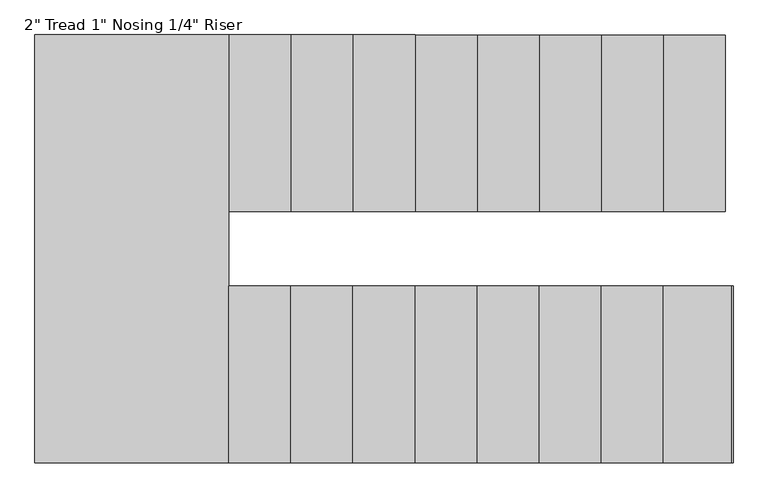
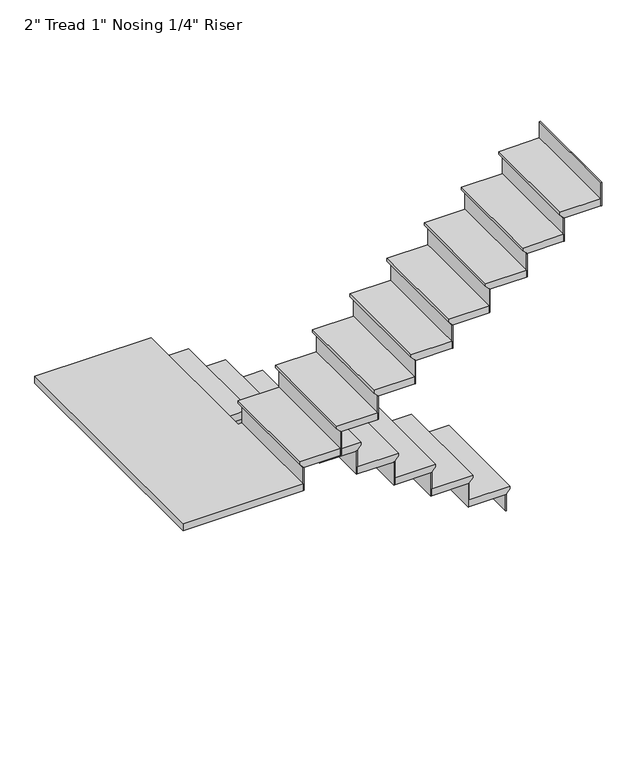
"""IFC4 building model written with IfcOpenShell, lengths in millimetres: stair flight geometry."""

from ifc_helpers import new_model, si_unit, origin, place, context, project, spatial, faceted_brep, source, transform, mapped, element, save


def stair_flight_94c6aef5(model_context):
    return source(origin(), model_context, "Body", "Brep", [
        faceted_brep([(-2118.1728655, 1192.5797121, 9292.8722222), (-2118.1728655, 1192.5797121, 9311.9222222), (-2118.1728655, 468.6797121, 9311.9222222), (-2118.1728655, 468.6797121, 9292.8722222), (-2143.5728655, 1192.5797121, 9267.4722222), (-2143.5728655, 468.6797121, 9267.4722222), (-2397.5728655, 1192.5797121, 9311.9222222), (-2397.5728655, 468.6797121, 9311.9222222), (-2143.5728655, 468.6797121, 9261.1222222), (-2397.5728655, 468.6797121, 9261.1222222), (-2397.5728655, 1192.5797121, 9261.1222222), (-2143.5728655, 1192.5797121, 9261.1222222)], [[[0, 1, 2, 3]], [[4, 0, 3, 5]], [[2, 1, 6, 7]], [[8, 9, 10, 11]], [[2, 7, 9, 8, 5, 3]], [[8, 11, 4, 5]], [[6, 1, 0, 4, 11, 10]], [[7, 6, 10, 9]]]),
        faceted_brep([(-2143.5728655, 1192.5797121, 9261.1222222), (-2143.5728655, 1192.5797121, 9144.0), (-2149.9228655, 1192.5797121, 9144.0), (-2149.9228655, 1192.5797121, 9261.1222222), (-2143.5728655, 468.6797121, 9261.1222222), (-2149.9228655, 468.6797121, 9261.1222222), (-2149.9228655, 468.6797121, 9144.0), (-2143.5728655, 468.6797121, 9144.0)], [[[0, 1, 2, 3]], [[4, 5, 6, 7]], [[1, 0, 4, 7]], [[2, 1, 7, 6]], [[3, 2, 6, 5]], [[0, 3, 5, 4]]]),
        faceted_brep([(-2397.5728655, 1192.5797121, 9429.0444444), (-2397.5728655, 1192.5797121, 9261.1222222), (-2403.9228655, 1192.5797121, 9261.1222222), (-2403.9228655, 1192.5797121, 9429.0444444), (-2397.5728655, 468.6797121, 9429.0444444), (-2403.9228655, 468.6797121, 9429.0444444), (-2403.9228655, 468.6797121, 9261.1222222), (-2397.5728655, 468.6797121, 9261.1222222)], [[[0, 1, 2, 3]], [[4, 5, 6, 7]], [[1, 0, 4, 7]], [[2, 1, 7, 6]], [[3, 2, 6, 5]], [[0, 3, 5, 4]]]),
        faceted_brep([(-2372.1728655, 468.6797121, 9479.8444444), (-2372.1728655, 1192.5797121, 9479.8444444), (-2651.5728655, 1192.5797121, 9479.8444444), (-2651.5728655, 468.6797121, 9479.8444444), (-2397.5728655, 468.6797121, 9429.0444444), (-2651.5728655, 468.6797121, 9429.0444444), (-2651.5728655, 1192.5797121, 9429.0444444), (-2397.5728655, 1192.5797121, 9429.0444444), (-2397.5728655, 468.6797121, 9435.3944444), (-2372.1728655, 468.6797121, 9460.7944444), (-2397.5728655, 1192.5797121, 9435.3944444), (-2372.1728655, 1192.5797121, 9460.7944444)], [[[0, 1, 2, 3]], [[4, 5, 6, 7]], [[0, 3, 5, 4, 8, 9]], [[4, 7, 10, 8]], [[2, 1, 11, 10, 7, 6]], [[3, 2, 6, 5]], [[11, 1, 0, 9]], [[10, 11, 9, 8]]]),
        faceted_brep([(-2651.5728655, 1192.5797121, 9596.9666667), (-2651.5728655, 1192.5797121, 9429.0444444), (-2657.9228655, 1192.5797121, 9429.0444444), (-2657.9228655, 1192.5797121, 9596.9666667), (-2651.5728655, 468.6797121, 9596.9666667), (-2657.9228655, 468.6797121, 9596.9666667), (-2657.9228655, 468.6797121, 9429.0444444), (-2651.5728655, 468.6797121, 9429.0444444)], [[[0, 1, 2, 3]], [[4, 5, 6, 7]], [[1, 0, 4, 7]], [[2, 1, 7, 6]], [[3, 2, 6, 5]], [[0, 3, 5, 4]]]),
        faceted_brep([(-2626.1728655, 468.6797121, 9647.7666667), (-2626.1728655, 1192.5797121, 9647.7666667), (-2905.5728655, 1192.5797121, 9647.7666667), (-2905.5728655, 468.6797121, 9647.7666667), (-2651.5728655, 468.6797121, 9596.9666667), (-2905.5728655, 468.6797121, 9596.9666667), (-2905.5728655, 1192.5797121, 9596.9666667), (-2651.5728655, 1192.5797121, 9596.9666667), (-2651.5728655, 468.6797121, 9603.3166667), (-2626.1728655, 468.6797121, 9628.7166667), (-2651.5728655, 1192.5797121, 9603.3166667), (-2626.1728655, 1192.5797121, 9628.7166667)], [[[0, 1, 2, 3]], [[4, 5, 6, 7]], [[0, 3, 5, 4, 8, 9]], [[4, 7, 10, 8]], [[2, 1, 11, 10, 7, 6]], [[3, 2, 6, 5]], [[11, 1, 0, 9]], [[10, 11, 9, 8]]]),
        faceted_brep([(-2905.5728655, 1192.5797121, 9764.8888889), (-2905.5728655, 1192.5797121, 9596.9666667), (-2911.9228655, 1192.5797121, 9596.9666667), (-2911.9228655, 1192.5797121, 9764.8888889), (-2905.5728655, 468.6797121, 9764.8888889), (-2911.9228655, 468.6797121, 9764.8888889), (-2911.9228655, 468.6797121, 9596.9666667), (-2905.5728655, 468.6797121, 9596.9666667)], [[[0, 1, 2, 3]], [[4, 5, 6, 7]], [[1, 0, 4, 7]], [[2, 1, 7, 6]], [[3, 2, 6, 5]], [[0, 3, 5, 4]]]),
        faceted_brep([(-2880.1728655, 468.6797121, 9815.6888889), (-2880.1728655, 1192.5797121, 9815.6888889), (-3159.5728655, 1192.5797121, 9815.6888889), (-3159.5728655, 468.6797121, 9815.6888889), (-2905.5728655, 468.6797121, 9764.8888889), (-3159.5728655, 468.6797121, 9764.8888889), (-3159.5728655, 1192.5797121, 9764.8888889), (-2905.5728655, 1192.5797121, 9764.8888889), (-2905.5728655, 468.6797121, 9771.2388889), (-2880.1728655, 468.6797121, 9796.6388889), (-2905.5728655, 1192.5797121, 9771.2388889), (-2880.1728655, 1192.5797121, 9796.6388889)], [[[0, 1, 2, 3]], [[4, 5, 6, 7]], [[0, 3, 5, 4, 8, 9]], [[4, 7, 10, 8]], [[2, 1, 11, 10, 7, 6]], [[3, 2, 6, 5]], [[11, 1, 0, 9]], [[10, 11, 9, 8]]]),
        faceted_brep([(-3159.5728655, 1192.5797121, 9932.8111111), (-3159.5728655, 1192.5797121, 9764.8888889), (-3165.9228655, 1192.5797121, 9764.8888889), (-3165.9228655, 1192.5797121, 9932.8111111), (-3159.5728655, 468.6797121, 9932.8111111), (-3165.9228655, 468.6797121, 9932.8111111), (-3165.9228655, 468.6797121, 9764.8888889), (-3159.5728655, 468.6797121, 9764.8888889)], [[[0, 1, 2, 3]], [[4, 5, 6, 7]], [[1, 0, 4, 7]], [[2, 1, 7, 6]], [[3, 2, 6, 5]], [[0, 3, 5, 4]]]),
        faceted_brep([(-3134.1728655, 468.6797121, 9983.6111111), (-3134.1728655, 1192.5797121, 9983.6111111), (-3413.5728655, 1192.5797121, 9983.6111111), (-3413.5728655, 468.6797121, 9983.6111111), (-3159.5728655, 468.6797121, 9932.8111111), (-3413.5728655, 468.6797121, 9932.8111111), (-3413.5728655, 1192.5797121, 9932.8111111), (-3159.5728655, 1192.5797121, 9932.8111111), (-3159.5728655, 468.6797121, 9939.1611111), (-3134.1728655, 468.6797121, 9964.5611111), (-3159.5728655, 1192.5797121, 9939.1611111), (-3134.1728655, 1192.5797121, 9964.5611111)], [[[0, 1, 2, 3]], [[4, 5, 6, 7]], [[0, 3, 5, 4, 8, 9]], [[4, 7, 10, 8]], [[2, 1, 11, 10, 7, 6]], [[3, 2, 6, 5]], [[11, 1, 0, 9]], [[10, 11, 9, 8]]]),
        faceted_brep([(-3413.5728655, 1192.5797121, 10100.7333333), (-3413.5728655, 1192.5797121, 9932.8111111), (-3419.9228655, 1192.5797121, 9932.8111111), (-3419.9228655, 1192.5797121, 10100.7333333), (-3413.5728655, 468.6797121, 10100.7333333), (-3419.9228655, 468.6797121, 10100.7333333), (-3419.9228655, 468.6797121, 9932.8111111), (-3413.5728655, 468.6797121, 9932.8111111)], [[[0, 1, 2, 3]], [[4, 5, 6, 7]], [[1, 0, 4, 7]], [[2, 1, 7, 6]], [[3, 2, 6, 5]], [[0, 3, 5, 4]]]),
        faceted_brep([(-3388.1728655, 468.6797121, 10151.5333333), (-3388.1728655, 1192.5797121, 10151.5333333), (-3667.5728655, 1192.5797121, 10151.5333333), (-3667.5728655, 468.6797121, 10151.5333333), (-3413.5728655, 468.6797121, 10100.7333333), (-3667.5728655, 468.6797121, 10100.7333333), (-3667.5728655, 1192.5797121, 10100.7333333), (-3413.5728655, 1192.5797121, 10100.7333333), (-3413.5728655, 468.6797121, 10107.0833333), (-3388.1728655, 468.6797121, 10132.4833333), (-3413.5728655, 1192.5797121, 10107.0833333), (-3388.1728655, 1192.5797121, 10132.4833333)], [[[0, 1, 2, 3]], [[4, 5, 6, 7]], [[0, 3, 5, 4, 8, 9]], [[4, 7, 10, 8]], [[2, 1, 11, 10, 7, 6]], [[3, 2, 6, 5]], [[11, 1, 0, 9]], [[10, 11, 9, 8]]]),
        faceted_brep([(-3667.5728655, 1192.5797121, 10268.6555556), (-3667.5728655, 1192.5797121, 10100.7333333), (-3673.9228655, 1192.5797121, 10100.7333333), (-3673.9228655, 1192.5797121, 10268.6555556), (-3667.5728655, 468.6797121, 10268.6555556), (-3673.9228655, 468.6797121, 10268.6555556), (-3673.9228655, 468.6797121, 10100.7333333), (-3667.5728655, 468.6797121, 10100.7333333)], [[[0, 1, 2, 3]], [[4, 5, 6, 7]], [[1, 0, 4, 7]], [[2, 1, 7, 6]], [[3, 2, 6, 5]], [[0, 3, 5, 4]]]),
        faceted_brep([(-3642.1728655, 468.6797121, 10319.4555556), (-3642.1728655, 1192.5797121, 10319.4555556), (-3921.5728655, 1192.5797121, 10319.4555556), (-3921.5728655, 468.6797121, 10319.4555556), (-3667.5728655, 468.6797121, 10268.6555556), (-3921.5728655, 468.6797121, 10268.6555556), (-3921.5728655, 1192.5797121, 10268.6555556), (-3667.5728655, 1192.5797121, 10268.6555556), (-3667.5728655, 468.6797121, 10275.0055556), (-3642.1728655, 468.6797121, 10300.4055556), (-3667.5728655, 1192.5797121, 10275.0055556), (-3642.1728655, 1192.5797121, 10300.4055556)], [[[0, 1, 2, 3]], [[4, 5, 6, 7]], [[0, 3, 5, 4, 8, 9]], [[4, 7, 10, 8]], [[2, 1, 11, 10, 7, 6]], [[3, 2, 6, 5]], [[11, 1, 0, 9]], [[10, 11, 9, 8]]]),
        faceted_brep([(-3921.5728655, 1192.5797121, 10436.5777778), (-3921.5728655, 1192.5797121, 10268.6555556), (-3927.9228655, 1192.5797121, 10268.6555556), (-3927.9228655, 1192.5797121, 10436.5777778), (-3921.5728655, 468.6797121, 10436.5777778), (-3927.9228655, 468.6797121, 10436.5777778), (-3927.9228655, 468.6797121, 10268.6555556), (-3921.5728655, 468.6797121, 10268.6555556)], [[[0, 1, 2, 3]], [[4, 5, 6, 7]], [[1, 0, 4, 7]], [[2, 1, 7, 6]], [[3, 2, 6, 5]], [[0, 3, 5, 4]]]),
        faceted_brep([(-3896.1728655, 468.6797121, 10487.3777778), (-3896.1728655, 1192.5797121, 10487.3777778), (-4175.5728655, 1192.5797121, 10487.3777778), (-4175.5728655, 468.6797121, 10487.3777778), (-3921.5728655, 468.6797121, 10436.5777778), (-4175.5728655, 468.6797121, 10436.5777778), (-4175.5728655, 1192.5797121, 10436.5777778), (-3921.5728655, 1192.5797121, 10436.5777778), (-3921.5728655, 468.6797121, 10442.9277778), (-3896.1728655, 468.6797121, 10468.3277778), (-3921.5728655, 1192.5797121, 10442.9277778), (-3896.1728655, 1192.5797121, 10468.3277778)], [[[0, 1, 2, 3]], [[4, 5, 6, 7]], [[0, 3, 5, 4, 8, 9]], [[4, 7, 10, 8]], [[2, 1, 11, 10, 7, 6]], [[3, 2, 6, 5]], [[11, 1, 0, 9]], [[10, 11, 9, 8]]]),
        faceted_brep([(-4175.5728655, 1192.5797121, 10604.5), (-4175.5728655, 1192.5797121, 10436.5777778), (-4181.9228655, 1192.5797121, 10436.5777778), (-4181.9228655, 1192.5797121, 10604.5), (-4175.5728655, 468.6797121, 10604.5), (-4181.9228655, 468.6797121, 10604.5), (-4181.9228655, 468.6797121, 10436.5777778), (-4175.5728655, 468.6797121, 10436.5777778)], [[[0, 1, 2, 3]], [[4, 5, 6, 7]], [[1, 0, 4, 7]], [[2, 1, 7, 6]], [[3, 2, 6, 5]], [[0, 3, 5, 4]]]),
        faceted_brep([(-4124.7728655, 163.8797121, 10655.3), (-4150.1728655, 163.8797121, 10655.3), (-4150.1728655, 1192.5797121, 10655.3), (-4943.9394105, 1192.5797121, 10655.3), (-4943.9394105, -560.0202879, 10655.3), (-4124.7728655, -560.0202879, 10655.3), (-4150.1728655, 163.8797121, 10604.5), (-4124.7728655, 163.8797121, 10604.5), (-4124.7728655, -560.0202879, 10604.5), (-4943.9394105, -560.0202879, 10604.5), (-4943.9394105, 1192.5797121, 10604.5), (-4175.5728655, 1192.5797121, 10604.5), (-4175.5728655, 468.6797121, 10604.5), (-4150.1728655, 468.6797121, 10604.5), (-4150.1728655, 468.6797121, 10636.25), (-4150.1728655, 1192.5797121, 10636.25), (-4175.5728655, 468.6797121, 10610.85), (-4175.5728655, 1192.5797121, 10610.85)], [[[0, 1, 2, 3, 4, 5]], [[6, 7, 8, 9, 10, 11, 12, 13]], [[1, 0, 7, 6]], [[2, 1, 6, 13, 14, 15]], [[13, 12, 16, 14]], [[12, 11, 17, 16]], [[3, 2, 15, 17, 11, 10]], [[4, 3, 10, 9]], [[5, 4, 9, 8]], [[0, 5, 8, 7]], [[17, 15, 14, 16]]]),
        faceted_brep([(-4124.7728655, -560.0202879, 10772.4222222), (-4124.7728655, -560.0202879, 10604.5), (-4118.4228655, -560.0202879, 10604.5), (-4118.4228655, -560.0202879, 10772.4222222), (-4124.7728655, 163.8797121, 10772.4222222), (-4118.4228655, 163.8797121, 10772.4222222), (-4118.4228655, 163.8797121, 10604.5), (-4124.7728655, 163.8797121, 10604.5)], [[[0, 1, 2, 3]], [[4, 5, 6, 7]], [[1, 0, 4, 7]], [[2, 1, 7, 6]], [[3, 2, 6, 5]], [[0, 3, 5, 4]]]),
        faceted_brep([(-4150.1728655, 163.8797121, 10823.2222222), (-4150.1728655, -560.0202879, 10823.2222222), (-3870.7728655, -560.0202879, 10823.2222222), (-3870.7728655, 163.8797121, 10823.2222222), (-4124.7728655, 163.8797121, 10772.4222222), (-3870.7728655, 163.8797121, 10772.4222222), (-3870.7728655, -560.0202879, 10772.4222222), (-4124.7728655, -560.0202879, 10772.4222222), (-4124.7728655, 163.8797121, 10778.7722222), (-4150.1728655, 163.8797121, 10804.1722222), (-4124.7728655, -560.0202879, 10778.7722222), (-4150.1728655, -560.0202879, 10804.1722222)], [[[0, 1, 2, 3]], [[4, 5, 6, 7]], [[0, 3, 5, 4, 8, 9]], [[4, 7, 10, 8]], [[2, 1, 11, 10, 7, 6]], [[3, 2, 6, 5]], [[11, 1, 0, 9]], [[10, 11, 9, 8]]]),
        faceted_brep([(-3870.7728655, -560.0202879, 10940.3444444), (-3870.7728655, -560.0202879, 10772.4222222), (-3864.4228655, -560.0202879, 10772.4222222), (-3864.4228655, -560.0202879, 10940.3444444), (-3870.7728655, 163.8797121, 10940.3444444), (-3864.4228655, 163.8797121, 10940.3444444), (-3864.4228655, 163.8797121, 10772.4222222), (-3870.7728655, 163.8797121, 10772.4222222)], [[[0, 1, 2, 3]], [[4, 5, 6, 7]], [[1, 0, 4, 7]], [[2, 1, 7, 6]], [[3, 2, 6, 5]], [[0, 3, 5, 4]]]),
        faceted_brep([(-3896.1728655, 163.8797121, 10991.1444444), (-3896.1728655, -560.0202879, 10991.1444444), (-3616.7728655, -560.0202879, 10991.1444444), (-3616.7728655, 163.8797121, 10991.1444444), (-3870.7728655, 163.8797121, 10940.3444444), (-3616.7728655, 163.8797121, 10940.3444444), (-3616.7728655, -560.0202879, 10940.3444444), (-3870.7728655, -560.0202879, 10940.3444444), (-3870.7728655, 163.8797121, 10946.6944444), (-3896.1728655, 163.8797121, 10972.0944444), (-3870.7728655, -560.0202879, 10946.6944444), (-3896.1728655, -560.0202879, 10972.0944444)], [[[0, 1, 2, 3]], [[4, 5, 6, 7]], [[0, 3, 5, 4, 8, 9]], [[4, 7, 10, 8]], [[2, 1, 11, 10, 7, 6]], [[3, 2, 6, 5]], [[11, 1, 0, 9]], [[10, 11, 9, 8]]]),
        faceted_brep([(-3616.7728655, -560.0202879, 11108.2666667), (-3616.7728655, -560.0202879, 10940.3444444), (-3610.4228655, -560.0202879, 10940.3444444), (-3610.4228655, -560.0202879, 11108.2666667), (-3616.7728655, 163.8797121, 11108.2666667), (-3610.4228655, 163.8797121, 11108.2666667), (-3610.4228655, 163.8797121, 10940.3444444), (-3616.7728655, 163.8797121, 10940.3444444)], [[[0, 1, 2, 3]], [[4, 5, 6, 7]], [[1, 0, 4, 7]], [[2, 1, 7, 6]], [[3, 2, 6, 5]], [[0, 3, 5, 4]]]),
        faceted_brep([(-3642.1728655, 163.8797121, 11159.0666667), (-3642.1728655, -560.0202879, 11159.0666667), (-3362.7728655, -560.0202879, 11159.0666667), (-3362.7728655, 163.8797121, 11159.0666667), (-3616.7728655, 163.8797121, 11108.2666667), (-3362.7728655, 163.8797121, 11108.2666667), (-3362.7728655, -560.0202879, 11108.2666667), (-3616.7728655, -560.0202879, 11108.2666667), (-3616.7728655, 163.8797121, 11114.6166667), (-3642.1728655, 163.8797121, 11140.0166667), (-3616.7728655, -560.0202879, 11114.6166667), (-3642.1728655, -560.0202879, 11140.0166667)], [[[0, 1, 2, 3]], [[4, 5, 6, 7]], [[0, 3, 5, 4, 8, 9]], [[4, 7, 10, 8]], [[2, 1, 11, 10, 7, 6]], [[3, 2, 6, 5]], [[11, 1, 0, 9]], [[10, 11, 9, 8]]]),
        faceted_brep([(-3362.7728655, -560.0202879, 11276.1888889), (-3362.7728655, -560.0202879, 11108.2666667), (-3356.4228655, -560.0202879, 11108.2666667), (-3356.4228655, -560.0202879, 11276.1888889), (-3362.7728655, 163.8797121, 11276.1888889), (-3356.4228655, 163.8797121, 11276.1888889), (-3356.4228655, 163.8797121, 11108.2666667), (-3362.7728655, 163.8797121, 11108.2666667)], [[[0, 1, 2, 3]], [[4, 5, 6, 7]], [[1, 0, 4, 7]], [[2, 1, 7, 6]], [[3, 2, 6, 5]], [[0, 3, 5, 4]]]),
        faceted_brep([(-3388.1728655, 163.8797121, 11326.9888889), (-3388.1728655, -560.0202879, 11326.9888889), (-3108.7728655, -560.0202879, 11326.9888889), (-3108.7728655, 163.8797121, 11326.9888889), (-3362.7728655, 163.8797121, 11276.1888889), (-3108.7728655, 163.8797121, 11276.1888889), (-3108.7728655, -560.0202879, 11276.1888889), (-3362.7728655, -560.0202879, 11276.1888889), (-3362.7728655, 163.8797121, 11282.5388889), (-3388.1728655, 163.8797121, 11307.9388889), (-3362.7728655, -560.0202879, 11282.5388889), (-3388.1728655, -560.0202879, 11307.9388889)], [[[0, 1, 2, 3]], [[4, 5, 6, 7]], [[0, 3, 5, 4, 8, 9]], [[4, 7, 10, 8]], [[2, 1, 11, 10, 7, 6]], [[3, 2, 6, 5]], [[11, 1, 0, 9]], [[10, 11, 9, 8]]]),
        faceted_brep([(-3108.7728655, -560.0202879, 11444.1111111), (-3108.7728655, -560.0202879, 11276.1888889), (-3102.4228655, -560.0202879, 11276.1888889), (-3102.4228655, -560.0202879, 11444.1111111), (-3108.7728655, 163.8797121, 11444.1111111), (-3102.4228655, 163.8797121, 11444.1111111), (-3102.4228655, 163.8797121, 11276.1888889), (-3108.7728655, 163.8797121, 11276.1888889)], [[[0, 1, 2, 3]], [[4, 5, 6, 7]], [[1, 0, 4, 7]], [[2, 1, 7, 6]], [[3, 2, 6, 5]], [[0, 3, 5, 4]]]),
        faceted_brep([(-3134.1728655, 163.8797121, 11494.9111111), (-3134.1728655, -560.0202879, 11494.9111111), (-2854.7728655, -560.0202879, 11494.9111111), (-2854.7728655, 163.8797121, 11494.9111111), (-3108.7728655, 163.8797121, 11444.1111111), (-2854.7728655, 163.8797121, 11444.1111111), (-2854.7728655, -560.0202879, 11444.1111111), (-3108.7728655, -560.0202879, 11444.1111111), (-3108.7728655, 163.8797121, 11450.4611111), (-3134.1728655, 163.8797121, 11475.8611111), (-3108.7728655, -560.0202879, 11450.4611111), (-3134.1728655, -560.0202879, 11475.8611111)], [[[0, 1, 2, 3]], [[4, 5, 6, 7]], [[0, 3, 5, 4, 8, 9]], [[4, 7, 10, 8]], [[2, 1, 11, 10, 7, 6]], [[3, 2, 6, 5]], [[11, 1, 0, 9]], [[10, 11, 9, 8]]]),
        faceted_brep([(-2854.7728655, -560.0202879, 11612.0333333), (-2854.7728655, -560.0202879, 11444.1111111), (-2848.4228655, -560.0202879, 11444.1111111), (-2848.4228655, -560.0202879, 11612.0333333), (-2854.7728655, 163.8797121, 11612.0333333), (-2848.4228655, 163.8797121, 11612.0333333), (-2848.4228655, 163.8797121, 11444.1111111), (-2854.7728655, 163.8797121, 11444.1111111)], [[[0, 1, 2, 3]], [[4, 5, 6, 7]], [[1, 0, 4, 7]], [[2, 1, 7, 6]], [[3, 2, 6, 5]], [[0, 3, 5, 4]]]),
        faceted_brep([(-2880.1728655, 163.8797121, 11662.8333333), (-2880.1728655, -560.0202879, 11662.8333333), (-2600.7728655, -560.0202879, 11662.8333333), (-2600.7728655, 163.8797121, 11662.8333333), (-2854.7728655, 163.8797121, 11612.0333333), (-2600.7728655, 163.8797121, 11612.0333333), (-2600.7728655, -560.0202879, 11612.0333333), (-2854.7728655, -560.0202879, 11612.0333333), (-2854.7728655, 163.8797121, 11618.3833333), (-2880.1728655, 163.8797121, 11643.7833333), (-2854.7728655, -560.0202879, 11618.3833333), (-2880.1728655, -560.0202879, 11643.7833333)], [[[0, 1, 2, 3]], [[4, 5, 6, 7]], [[0, 3, 5, 4, 8, 9]], [[4, 7, 10, 8]], [[2, 1, 11, 10, 7, 6]], [[3, 2, 6, 5]], [[11, 1, 0, 9]], [[10, 11, 9, 8]]]),
        faceted_brep([(-2600.7728655, -560.0202879, 11779.9555556), (-2600.7728655, -560.0202879, 11612.0333333), (-2594.4228655, -560.0202879, 11612.0333333), (-2594.4228655, -560.0202879, 11779.9555556), (-2600.7728655, 163.8797121, 11779.9555556), (-2594.4228655, 163.8797121, 11779.9555556), (-2594.4228655, 163.8797121, 11612.0333333), (-2600.7728655, 163.8797121, 11612.0333333)], [[[0, 1, 2, 3]], [[4, 5, 6, 7]], [[1, 0, 4, 7]], [[2, 1, 7, 6]], [[3, 2, 6, 5]], [[0, 3, 5, 4]]]),
        faceted_brep([(-2626.1728655, 163.8797121, 11830.7555556), (-2626.1728655, -560.0202879, 11830.7555556), (-2346.7728655, -560.0202879, 11830.7555556), (-2346.7728655, 163.8797121, 11830.7555556), (-2600.7728655, 163.8797121, 11779.9555556), (-2346.7728655, 163.8797121, 11779.9555556), (-2346.7728655, -560.0202879, 11779.9555556), (-2600.7728655, -560.0202879, 11779.9555556), (-2600.7728655, 163.8797121, 11786.3055556), (-2626.1728655, 163.8797121, 11811.7055556), (-2600.7728655, -560.0202879, 11786.3055556), (-2626.1728655, -560.0202879, 11811.7055556)], [[[0, 1, 2, 3]], [[4, 5, 6, 7]], [[0, 3, 5, 4, 8, 9]], [[4, 7, 10, 8]], [[2, 1, 11, 10, 7, 6]], [[3, 2, 6, 5]], [[11, 1, 0, 9]], [[10, 11, 9, 8]]]),
        faceted_brep([(-2346.7728655, -560.0202879, 11947.8777778), (-2346.7728655, -560.0202879, 11779.9555556), (-2340.4228655, -560.0202879, 11779.9555556), (-2340.4228655, -560.0202879, 11947.8777778), (-2346.7728655, 163.8797121, 11947.8777778), (-2340.4228655, 163.8797121, 11947.8777778), (-2340.4228655, 163.8797121, 11779.9555556), (-2346.7728655, 163.8797121, 11779.9555556)], [[[0, 1, 2, 3]], [[4, 5, 6, 7]], [[1, 0, 4, 7]], [[2, 1, 7, 6]], [[3, 2, 6, 5]], [[0, 3, 5, 4]]]),
        faceted_brep([(-2092.7728655, -560.0202879, 12115.8), (-2092.7728655, -560.0202879, 11947.8777778), (-2086.4228655, -560.0202879, 11947.8777778), (-2086.4228655, -560.0202879, 12115.8), (-2092.7728655, 163.8797121, 12115.8), (-2086.4228655, 163.8797121, 12115.8), (-2086.4228655, 163.8797121, 11947.8777778), (-2092.7728655, 163.8797121, 11947.8777778)], [[[0, 1, 2, 3]], [[4, 5, 6, 7]], [[1, 0, 4, 7]], [[2, 1, 7, 6]], [[3, 2, 6, 5]], [[0, 3, 5, 4]]]),
        faceted_brep([(-2372.1728655, 163.8797121, 11998.6777778), (-2372.1728655, -560.0202879, 11998.6777778), (-2092.7728655, -560.0202879, 11998.6777778), (-2092.7728655, 163.8797121, 11998.6777778), (-2346.7728655, 163.8797121, 11947.8777778), (-2092.7728655, 163.8797121, 11947.8777778), (-2092.7728655, -560.0202879, 11947.8777778), (-2346.7728655, -560.0202879, 11947.8777778), (-2346.7728655, 163.8797121, 11954.2277778), (-2372.1728655, 163.8797121, 11979.6277778), (-2346.7728655, -560.0202879, 11954.2277778), (-2372.1728655, -560.0202879, 11979.6277778)], [[[0, 1, 2, 3]], [[4, 5, 6, 7]], [[0, 3, 5, 4, 8, 9]], [[4, 7, 10, 8]], [[2, 1, 11, 10, 7, 6]], [[3, 2, 6, 5]], [[11, 1, 0, 9]], [[10, 11, 9, 8]]]),
    ])


if __name__ == "__main__":
    model = new_model("IFC4")
    model_context = context("Model", 3, world=origin())
    ifc_project = project(units=[si_unit("LENGTHUNIT", "METRE", prefix="MILLI")], contexts=[model_context])
    site = spatial("IfcSite", under=ifc_project)
    building = spatial("IfcBuilding", under=site)
    placement = place(None, origin())
    stair_flight_shape = stair_flight_94c6aef5(model_context)
    element("IfcStairFlight", 1, ObjectType="2\" Tread 1\" Nosing 1/4\" Riser", at=placement, inside=building, context=model_context, shape_type="MappedRepresentation", body=[
        mapped(stair_flight_shape, transform((0.0, 0.0, 0.0), x_axis=(1.0, 0.0, 0.0), y_axis=(0.0, 1.0, 0.0), z_axis=(0.0, 0.0, 1.0))),
    ])
    save(model, "model.ifc")
